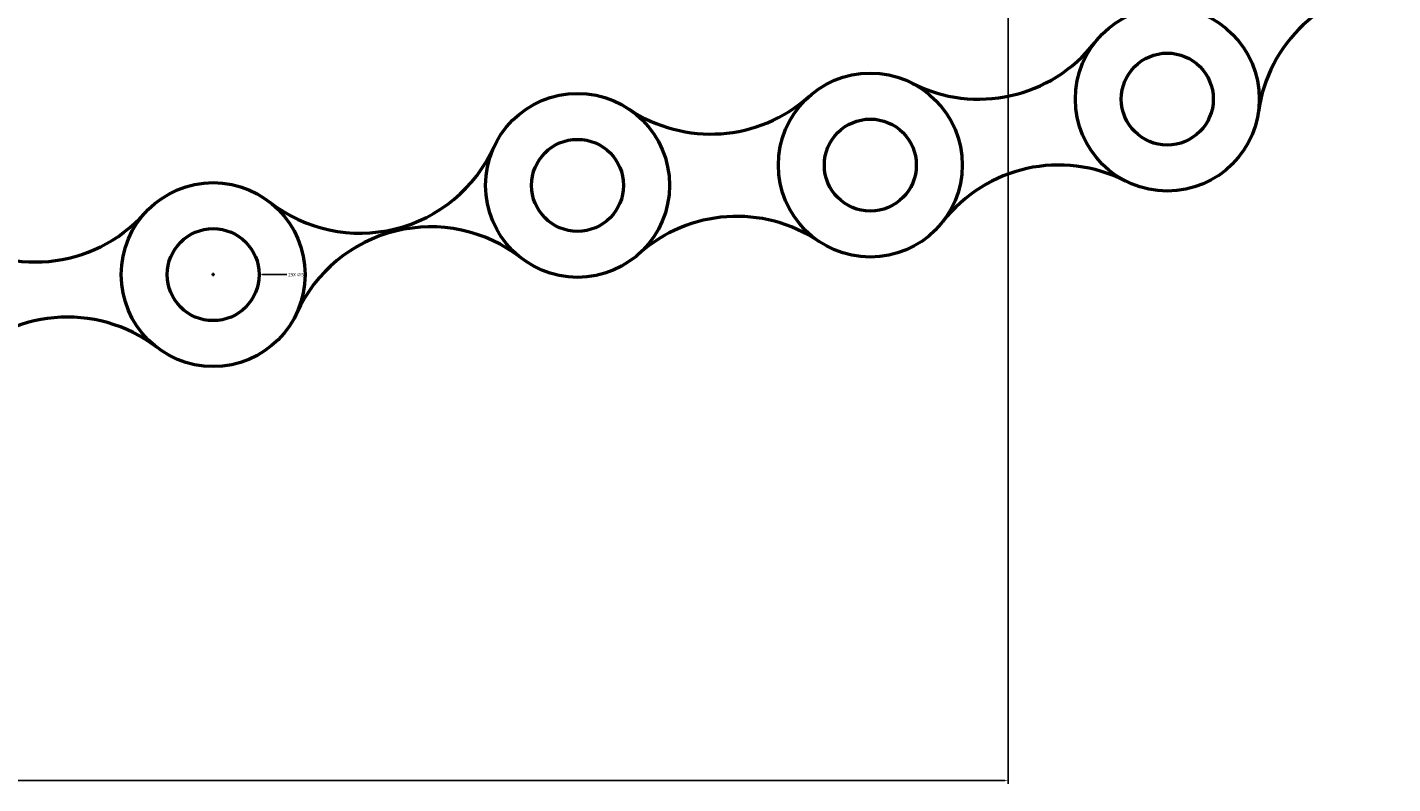
# Model space of a CAD drawing. Units: inches. Extents: x 413 to 622, y 326 to 447.
# Tile 10 of 15: x 539 to 614, y 326 to 367. Entities that reach past the tile are written whole.
import ezdxf

# ---------------------------------------------------------------- set-up
doc = ezdxf.new("R2010")
doc.units = ezdxf.units.IN
doc.header["$MEASUREMENT"] = 0
doc.layers.add('M-DIMS', color=2, linetype='Continuous', lineweight=18)
doc.layers.add('M-OUTL', color=7, linetype='Continuous', lineweight=50)
doc.styles.get("Standard").update_dxf_attribs({"font": 'arial.ttf'})
doc.dimstyles.get("Standard").update_dxf_attribs({"dimtxt": 0.18, "dimasz": 0.18, "dimexe": 0.18, "dimexo": 0.0625, "dimgap": 0.09, "dimtad": 0, "dimtih": 1, "dimtoh": 1, "dimdec": 4, "dimzin": 0, "dimdsep": 46, "dimtxsty": 'Standard', "dimcen": 0.09, "dimadec": 0, "dimazin": 0, "dimtfac": 1, "dimtdec": 4, "dimtofl": 0, "dimtmove": 0, "dimatfit": 3, "dimfxl": 1, "dimtolj": 1, "dimtzin": 0, "dimarcsym": 0})

# ---------------------------------------------------------------- blocks, each defined once
blk = doc.blocks.new('CHAIN-ROLLER-PIN')
for radius in [5, 2.5]:
    blk.add_circle((5, 5), radius)
blk = doc.blocks.new('CHAIN-LINK-WAIST-P17_664')
for centre, start, end in [((6.624, 13.651), 221.93853, 307.52912), ((4.873, -5.347), 41.93853, 127.52912)]:
    blk.add_arc(centre, 8, start, end)
blk = doc.blocks.new('CHAIN-LINK-WAIST-P20_400')
for centre, start, end in [((8.752, 12.333), 204.55472, 307.92191), ((4.917, -3.325), 24.55472, 127.92191)]:
    blk.add_arc(centre, 8, start, end)
blk = doc.blocks.new('*D12')
at = {"layer": 'Defpoints', "color": 0, "transparency": 16777216}
for p in [(472.684, 386.392), (592.684, 386.392), (592.684, 326.361)]:
    blk.add_point(p, dxfattribs=at)
at = {"layer": 'M-DIMS', "color": 0, "lineweight": -2, "transparency": 16777216}
for p, q in [((472.684, 386.329), (472.684, 326.181)), ((592.684, 386.329), (592.684, 326.181)), ((472.864, 326.361), (532.404, 326.361)), ((592.504, 326.361), (532.964, 326.361))]:
    blk.add_line(p, q, dxfattribs=at)
at = {"layer": 'M-DIMS', "color": 0, "transparency": 16777216}
for points in [[(472.864, 326.391), (472.864, 326.331), (472.684, 326.361)], [(592.504, 326.391), (592.504, 326.331), (592.684, 326.361)]]:
    blk.add_solid(points, dxfattribs=at)
at = {"layer": 'M-DIMS', "color": 0, "transparency": 16777216, "insert": (532.684, 326.361), "char_height": 0.18, "attachment_point": 5}
blk.add_mtext('\\A1;120', dxfattribs=at)
blk = doc.blocks.new('*D32')
at = {"layer": 'Defpoints', "color": 0, "transparency": 16777216}
for p in [(546.952, 353.846), (551.952, 353.845)]:
    blk.add_point(p, dxfattribs=at)
at = {"layer": 'M-DIMS', "color": 0, "lineweight": -2, "transparency": 16777216}
for p, q in [((549.362, 353.845), (549.542, 353.845)), ((549.452, 353.755), (549.452, 353.935)), ((553.452, 353.845), (552.132, 353.845))]:
    blk.add_line(p, q, dxfattribs=at)
at = {"layer": 'M-DIMS', "color": 0, "transparency": 16777216}
blk.add_solid([(552.132, 353.875), (552.132, 353.815), (551.952, 353.845)], dxfattribs=at)
at = {"layer": 'M-DIMS', "color": 0, "transparency": 16777216, "insert": (553.96, 353.845), "char_height": 0.18, "attachment_point": 5}
blk.add_mtext('\\A1;29X ∅5', dxfattribs=at)

msp = doc.modelspace()

# ---------------------------------------------------------------- linework, layer by layer
at = {"layer": 'M-OUTL'}
msp.add_circle((549.4524, 353.8455), 2.5, dxfattribs=at)
for centre, start, end in [((614.2144, 361.5964), 94.435125, 172.089592), ((591.0891, 371.3829), 243.003746, 322.034605), ((576.5191, 369.487), 236.089247, 311.823764), ((595.437, 351.802), 63.003746, 142.034605), ((577.9353, 349.0106), 56.089247, 131.823764)]:
    msp.add_arc(centre, 8, start, end, dxfattribs=at)

# ---------------------------------------------------------------- block references
for p in [(596.3385, 358.386), (580.1884, 354.7999), (564.2668, 353.6987), (544.4528, 348.846)]:
    msp.add_blockref('CHAIN-ROLLER-PIN', p, dxfattribs=at)
for name, p, rotation in [('CHAIN-LINK-WAIST-P20_400', (555.3799, 349.1192), 27.52337274548788), ('CHAIN-LINK-WAIST-P17_664', (545.5506, 358.1679), 190.5323476777275)]:
    msp.add_blockref(name, p, dxfattribs=dict(at, rotation=rotation))

# ---------------------------------------------------------------- dimensions: what is measured, and where the dimension line sits
at = {"layer": 'M-DIMS'}
dim = msp.add_linear_dim(base=(592.6836, 326.361), p1=(472.6836, 386.3915), p2=(592.6836, 386.3915), dimstyle='Standard', override={"dimdec": 0, "dimlfac": 1, "dimrnd": 0, "dimzin": 0, "dimdsep": 46, "dimlunit": 2}, dxfattribs=at)
dim.commit()
dim.dimension.update_dxf_attribs({"geometry": '*D12', "text_midpoint": (532.6836, 326.361)})
dim = msp.add_diameter_dim_2p(p1=(546.9524, 353.846), p2=(551.9524, 353.845), text='29X <>', dimstyle='Standard', override={"dimdec": 0, "dimlfac": 1, "dimrnd": 0, "dimzin": 0, "dimdsep": 46, "dimlunit": 2}, dxfattribs=at)
dim.commit()
dim.dimension.update_dxf_attribs({"geometry": '*D32', "text_midpoint": (553.4524, 353.8447), "dimtype": 163})

doc.saveas('drawing.dxf')
